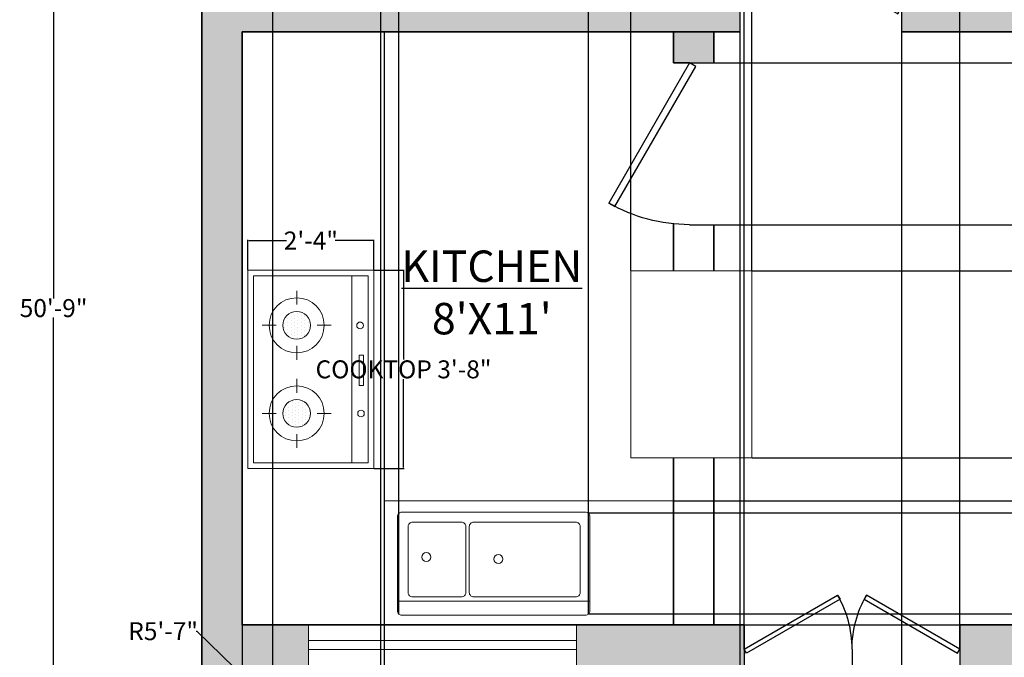
# Model space of a CAD drawing. Units: inches. Extents: x -37 to 408, y -619 to 75.
# Tile 2 of 4: x -37 to 182, y -354 to -212. Entities that reach past the tile are written whole.
import ezdxf

# ---------------------------------------------------------------- set-up
doc = ezdxf.new("R2010")
doc.units = ezdxf.units.IN
doc.header["$MEASUREMENT"] = 0
for name, color, linetype, lineweight in [('A-ANNO-DIMS', 2, 'Continuous', 18), ('A-AREA-IDEN', 7, 'Continuous', 25), ('A-DOOR', 4, 'Continuous', 25), ('A-EQPM', 9, 'Continuous', 18), ('A-FLOR-CASE', 8, 'Continuous', 18), ('A-FLOR-FIXT', 9, 'Continuous', 18), ('A-GLAZ', 4, 'Continuous', 18), ('A-WALL', 7, 'Continuous', 35), ('A-WALL-PATT', 16, 'Continuous', 13)]:
    doc.layers.add(name, color=color, linetype=linetype, lineweight=lineweight)
doc.styles.get("Standard").update_dxf_attribs({"font": 'arial.ttf'})
doc.dimstyles.get("Standard").update_dxf_attribs({"dimtxt": 4, "dimasz": 0.18, "dimexe": 0.18, "dimexo": 0.0625, "dimgap": 0.09, "dimtad": 0, "dimtih": 1, "dimtoh": 1, "dimdec": 1, "dimzin": 0, "dimdsep": 46, "dimlunit": 4, "dimtxsty": 'Standard', "dimcen": 0.09, "dimadec": 0, "dimazin": 0, "dimtfac": 1, "dimtdec": 1, "dimtofl": 0, "dimtmove": 0, "dimatfit": 3, "dimfxl": 1, "dimtolj": 1, "dimtzin": 0, "dimarcsym": 0})

# ---------------------------------------------------------------- blocks, each defined once
blk = doc.blocks.new('*U2')
for p, q in [((0, 0), (0, -6)), ((40, 0), (40, -6))]:
    blk.add_line(p, q)
blk.add_lwpolyline([(0, 0), (34.64, 20), (35.52, 18.48), (0.87, -1.52)], close=True)
blk.add_arc((0, 0), 40, 0, 30)
blk = doc.blocks.new('A$C475E21CF')
for p, q in [((0, 444.5), (0, 0)), ((0, 444.5), (699.9, 444.5)), ((19.4, 425), (19.4, 19.4)), ((19.4, 425), (680.5, 425)), ((680.5, 425), (680.5, 19.4)), ((699.9, 444.5), (699.9, 0)), ((194.5, 393.9), (194.5, 345.2)), ((505.4, 393.9), (505.4, 345.2)), ((498.4, 316.6), (498.4, 316.6)), ((510.6, 316.6), (510.6, 316.6)), ((522.7, 316.6), (522.7, 316.6)), ((160.9, 288.4), (160.9, 288.4)), ((166.9, 300.5), (166.9, 300.5)), ((173, 288.4), (173, 288.4)), ((179.1, 300.5), (179.1, 300.5)), ((185.2, 312.7), (185.2, 312.7)), ((185.2, 288.4), (185.2, 288.4)), ((191.2, 300.5), (191.2, 300.5)), ((197.3, 312.7), (197.3, 312.7)), ((197.3, 288.4), (197.3, 288.4)), ((203.4, 300.5), (203.4, 300.5)), ((209.5, 312.7), (209.5, 312.7)), ((209.5, 288.4), (209.5, 288.4)), ((215.6, 300.5), (215.6, 300.5)), ((221.6, 288.4), (221.6, 288.4)), ((227.7, 300.5), (227.7, 300.5)), ((233.8, 288.4), (233.8, 288.4)), ((468, 280.2), (468, 280.2)), ((474.1, 292.3), (474.1, 292.3)), ((480.2, 304.5), (480.2, 304.5)), ((480.2, 280.2), (480.2, 280.2)), ((486.3, 292.3), (486.3, 292.3)), ((492.3, 304.5), (492.3, 304.5)), ((492.3, 280.2), (492.3, 280.2)), ((498.4, 292.3), (498.4, 292.3)), ((504.5, 304.5), (504.5, 304.5)), ((504.5, 280.2), (504.5, 280.2)), ((510.6, 292.3), (510.6, 292.3)), ((516.7, 304.5), (516.7, 304.5)), ((516.7, 280.2), (516.7, 280.2)), ((522.7, 292.3), (522.7, 292.3)), ((528.8, 304.5), (528.8, 304.5)), ((528.8, 280.2), (528.8, 280.2)), ((534.9, 292.3), (534.9, 292.3)), ((541, 304.5), (541, 304.5)), ((541, 280.2), (541, 280.2)), ((547, 292.3), (547, 292.3)), ((553.1, 280.2), (553.1, 280.2)), ((72.9, 272.3), (121.6, 272.3)), ((148.7, 264.1), (148.7, 264.1)), ((154.8, 276.2), (154.8, 276.2)), ((154.8, 251.9), (154.8, 251.9)), ((160.9, 264.1), (160.9, 264.1)), ((166.9, 276.2), (166.9, 276.2)), ((166.9, 251.9), (166.9, 251.9)), ((173, 264.1), (173, 264.1)), ((179.1, 276.2), (179.1, 276.2)), ((179.1, 251.9), (179.1, 251.9)), ((185.2, 264.1), (185.2, 264.1)), ((191.2, 276.2), (191.2, 276.2)), ((191.2, 251.9), (191.2, 251.9)), ((197.3, 264.1), (197.3, 264.1)), ((203.4, 276.2), (203.4, 276.2)), ((203.4, 251.9), (203.4, 251.9)), ((209.5, 264.1), (209.5, 264.1)), ((215.6, 276.2), (215.6, 276.2)), ((215.6, 251.9), (215.6, 251.9)), ((221.6, 264.1), (221.6, 264.1)), ((227.7, 276.2), (227.7, 276.2)), ((227.7, 251.9), (227.7, 251.9)), ((233.8, 264.1), (233.8, 264.1)), ((239.9, 276.2), (239.9, 276.2)), ((239.9, 251.9), (239.9, 251.9)), ((267.4, 272.3), (316, 272.3)), ((383.9, 272.3), (432.5, 272.3)), ((462, 268), (462, 268)), ((468, 255.9), (468, 255.9)), ((474.1, 268), (474.1, 268)), ((474.1, 243.7), (474.1, 243.7)), ((480.2, 255.9), (480.2, 255.9)), ((486.3, 268), (486.3, 268)), ((486.3, 243.7), (486.3, 243.7)), ((492.3, 255.9), (492.3, 255.9)), ((498.4, 268), (498.4, 268)), ((498.4, 243.7), (498.4, 243.7)), ((504.5, 255.9), (504.5, 255.9)), ((510.6, 268), (510.6, 268)), ((510.6, 243.7), (510.6, 243.7)), ((516.7, 255.9), (516.7, 255.9)), ((522.7, 268), (522.7, 268)), ((522.7, 243.7), (522.7, 243.7)), ((528.8, 255.9), (528.8, 255.9)), ((534.9, 268), (534.9, 268)), ((534.9, 243.7), (534.9, 243.7)), ((541, 255.9), (541, 255.9)), ((547, 268), (547, 268)), ((547, 243.7), (547, 243.7)), ((553.1, 255.9), (553.1, 255.9)), ((578.4, 272.3), (627, 272.3)), ((160.9, 239.8), (160.9, 239.8)), ((173, 239.8), (173, 239.8)), ((179.1, 227.6), (179.1, 227.6)), ((185.2, 239.8), (185.2, 239.8)), ((191.2, 227.6), (191.2, 227.6)), ((197.3, 239.8), (197.3, 239.8)), ((203.4, 227.6), (203.4, 227.6)), ((209.5, 239.8), (209.5, 239.8)), ((215.6, 227.6), (215.6, 227.6)), ((221.6, 239.8), (221.6, 239.8)), ((233.8, 239.8), (233.8, 239.8)), ((492.3, 231.5), (492.3, 231.5)), ((504.5, 231.5), (504.5, 231.5)), ((516.7, 231.5), (516.7, 231.5)), ((528.8, 231.5), (528.8, 231.5)), ((194.5, 199.4), (194.5, 150.8)), ((505.4, 199.4), (505.4, 150.8)), ((19.4, 77.8), (680.5, 77.8)), ((293.4, 51.9), (400.6, 51.9)), ((293.4, 36.5), (293.4, 51.9)), ((400.6, 36.5), (293.4, 36.5)), ((400.6, 51.9), (400.6, 36.5)), ((0, 0), (699.9, 0)), ((19.4, 19.4), (680.5, 19.4))]:
    blk.add_line(p, q)
for centre, radius in [((194.5, 272.3), 97.2), ((505.4, 272.3), 97.2), ((194.5, 272.3), 48.6), ((505.4, 272.3), 48.6), ((193.9, 45.1), 11.7), ((505.2, 48.5), 11.7)]:
    blk.add_circle(centre, radius)
blk = doc.blocks.new('*D22')
at = {"layer": 'A-ANNO-DIMS', "color": 0, "lineweight": -2, "transparency": 16777216}
for p, q in [((41.93, -267.46), (48.67, -267.46)), ((48.49, -267.64), (48.49, -287.36)), ((48.49, -311.4), (48.49, -291.68)), ((41.93, -311.58), (48.67, -311.58))]:
    blk.add_line(p, q, dxfattribs=at)
at = {"layer": 'A-ANNO-DIMS', "color": 0, "transparency": 16777216}
for points in [[(48.46, -267.64), (48.52, -267.64), (48.49, -267.46)], [(48.46, -311.4), (48.52, -311.4), (48.49, -311.58)]]:
    blk.add_solid(points, dxfattribs=at)
at = {"layer": 'Defpoints', "color": 0, "transparency": 16777216}
for p in [(41.87, -267.46), (48.49, -267.46), (41.87, -311.58)]:
    blk.add_point(p, dxfattribs=at)
at = {"layer": 'A-ANNO-DIMS', "color": 0, "transparency": 16777216, "insert": (48.49, -289.52), "char_height": 4, "attachment_point": 5}
blk.add_mtext('\\A1;COOKTOP 3\'-8"', dxfattribs=at)
blk = doc.blocks.new('*D23')
at = {"layer": 'A-ANNO-DIMS', "color": 0, "lineweight": -2, "transparency": 16777216}
for p, q in [((13.85, -267.39), (13.85, -260.66)), ((14.03, -260.84), (22.42, -260.84)), ((41.69, -260.84), (33.3, -260.84)), ((41.87, -267.39), (41.87, -260.66))]:
    blk.add_line(p, q, dxfattribs=at)
at = {"layer": 'A-ANNO-DIMS', "color": 0, "transparency": 16777216}
for points in [[(14.03, -260.81), (14.03, -260.87), (13.85, -260.84)], [(41.69, -260.81), (41.69, -260.87), (41.87, -260.84)]]:
    blk.add_solid(points, dxfattribs=at)
at = {"layer": 'Defpoints', "color": 0, "transparency": 16777216}
for p in [(13.85, -260.84), (13.85, -267.46), (41.87, -267.46)]:
    blk.add_point(p, dxfattribs=at)
at = {"layer": 'A-ANNO-DIMS', "color": 0, "transparency": 16777216, "insert": (27.86, -260.84), "char_height": 4, "attachment_point": 5}
blk.add_mtext('\\A1;2\'-4"', dxfattribs=at)
blk = doc.blocks.new('*D28')
at = {"layer": 'A-ANNO-DIMS', "color": 0, "lineweight": -2, "transparency": 16777216}
for p, q in [((3.52, 28.62), (-29.6, 28.62)), ((-29.42, 28.44), (-29.42, -273.74)), ((-29.42, -580.2), (-29.42, -278.01)), ((3.52, -580.38), (-29.6, -580.38))]:
    blk.add_line(p, q, dxfattribs=at)
at = {"layer": 'A-ANNO-DIMS', "color": 0, "transparency": 16777216}
for points in [[(-29.45, 28.44), (-29.39, 28.44), (-29.42, 28.62)], [(-29.45, -580.2), (-29.39, -580.2), (-29.42, -580.38)]]:
    blk.add_solid(points, dxfattribs=at)
at = {"layer": 'Defpoints', "color": 0, "transparency": 16777216}
for p in [(-29.42, 28.62), (3.58, 28.62), (3.58, -580.38)]:
    blk.add_point(p, dxfattribs=at)
at = {"layer": 'A-ANNO-DIMS', "color": 0, "transparency": 16777216, "insert": (-29.42, -275.88), "char_height": 4, "attachment_point": 5}
blk.add_mtext('\\A1;50\'-9"', dxfattribs=at)
blk = doc.blocks.new('*D34')
at = {"layer": 'A-ANNO-DIMS', "color": 0, "lineweight": -2, "transparency": 16777216}
for p, q in [((124.36, -346.31), (124.36, 69.37)), ((124.54, 69.19), (142.88, 69.19)), ((172.18, 69.19), (153.85, 69.19)), ((172.36, -346.31), (172.36, 69.37))]:
    blk.add_line(p, q, dxfattribs=at)
at = {"layer": 'A-ANNO-DIMS', "color": 0, "transparency": 16777216}
for points in [[(124.54, 69.22), (124.54, 69.16), (124.36, 69.19)], [(172.18, 69.22), (172.18, 69.16), (172.36, 69.19)]]:
    blk.add_solid(points, dxfattribs=at)
at = {"layer": 'Defpoints', "color": 0, "transparency": 16777216}
for p in [(172.36, 69.19), (124.36, -346.38), (172.36, -346.38)]:
    blk.add_point(p, dxfattribs=at)
at = {"layer": 'A-ANNO-DIMS', "color": 0, "transparency": 16777216, "insert": (148.36, 69.19), "char_height": 4, "attachment_point": 5}
blk.add_mtext('\\A1;4\'-0"', dxfattribs=at)
blk = doc.blocks.new('*D37')
at = {"layer": 'A-ANNO-DIMS', "color": 0, "lineweight": -2, "transparency": 16777216}
for p, q in [((12.58, -214.44), (12.58, -613.56)), ((44.21, -214.44), (44.21, -613.56)), ((12.76, -613.38), (18.3, -613.38)), ((44.03, -613.38), (38.5, -613.38))]:
    blk.add_line(p, q, dxfattribs=at)
at = {"layer": 'A-ANNO-DIMS', "color": 0, "transparency": 16777216}
for points in [[(12.76, -613.35), (12.76, -613.41), (12.58, -613.38)], [(44.03, -613.35), (44.03, -613.41), (44.21, -613.38)]]:
    blk.add_solid(points, dxfattribs=at)
at = {"layer": 'Defpoints', "color": 0, "transparency": 16777216}
for p in [(12.58, -214.38), (44.21, -214.38), (44.21, -613.38)]:
    blk.add_point(p, dxfattribs=at)
at = {"layer": 'A-ANNO-DIMS', "color": 0, "transparency": 16777216, "insert": (28.4, -613.38), "char_height": 4, "attachment_point": 5}
blk.add_mtext('\\A1;2\'-7 1/2"', dxfattribs=at)
blk = doc.blocks.new('*D38')
at = {"layer": 'A-ANNO-DIMS', "color": 0, "lineweight": -2, "transparency": 16777216}
for p, q in [((123.34, -214.44), (123.34, -613.56)), ((159.34, -214.44), (159.34, -613.56)), ((123.52, -613.38), (135.93, -613.38)), ((159.16, -613.38), (146.74, -613.38))]:
    blk.add_line(p, q, dxfattribs=at)
at = {"layer": 'A-ANNO-DIMS', "color": 0, "transparency": 16777216}
for points in [[(123.52, -613.35), (123.52, -613.41), (123.34, -613.38)], [(159.16, -613.35), (159.16, -613.41), (159.34, -613.38)]]:
    blk.add_solid(points, dxfattribs=at)
at = {"layer": 'Defpoints', "color": 0, "transparency": 16777216}
for p in [(123.34, -214.38), (159.34, -214.38), (159.34, -613.38)]:
    blk.add_point(p, dxfattribs=at)
at = {"layer": 'A-ANNO-DIMS', "color": 0, "transparency": 16777216, "insert": (141.34, -613.38), "char_height": 4, "attachment_point": 5}
blk.add_mtext('\\A1;3\'-0"', dxfattribs=at)
blk = doc.blocks.new('*D39')
at = {"layer": 'A-ANNO-DIMS', "color": 0, "lineweight": -2, "transparency": 16777216}
for p, q in [((19.34, -49.44), (19.34, -613.56)), ((43.34, -49.44), (43.34, -613.56)), ((19.52, -613.38), (25.9, -613.38)), ((43.16, -613.38), (36.78, -613.38))]:
    blk.add_line(p, q, dxfattribs=at)
at = {"layer": 'A-ANNO-DIMS', "color": 0, "transparency": 16777216}
for points in [[(19.52, -613.35), (19.52, -613.41), (19.34, -613.38)], [(43.16, -613.35), (43.16, -613.41), (43.34, -613.38)]]:
    blk.add_solid(points, dxfattribs=at)
at = {"layer": 'Defpoints', "color": 0, "transparency": 16777216}
for p in [(19.34, -49.38), (43.34, -49.38), (43.34, -613.38)]:
    blk.add_point(p, dxfattribs=at)
at = {"layer": 'A-ANNO-DIMS', "color": 0, "transparency": 16777216, "insert": (31.34, -613.38), "char_height": 4, "attachment_point": 5}
blk.add_mtext('\\A1;2\'-0"', dxfattribs=at)
blk = doc.blocks.new('*D43')
at = {"layer": 'A-ANNO-DIMS', "color": 0, "lineweight": -2, "transparency": 16777216}
for p, q in [((47.42, -343.92), (47.42, 69.37)), ((47.6, 69.19), (58.49, 69.19)), ((89.51, 69.19), (78.62, 69.19)), ((89.69, -343.92), (89.69, 69.37))]:
    blk.add_line(p, q, dxfattribs=at)
at = {"layer": 'A-ANNO-DIMS', "color": 0, "transparency": 16777216}
for points in [[(47.6, 69.22), (47.6, 69.16), (47.42, 69.19)], [(89.51, 69.22), (89.51, 69.16), (89.69, 69.19)]]:
    blk.add_solid(points, dxfattribs=at)
at = {"layer": 'Defpoints', "color": 0, "transparency": 16777216}
for p in [(89.69, 69.19), (47.42, -343.98), (89.69, -343.98)]:
    blk.add_point(p, dxfattribs=at)
at = {"layer": 'A-ANNO-DIMS', "color": 0, "transparency": 16777216, "insert": (68.55, 69.19), "char_height": 4, "attachment_point": 5}
blk.add_mtext('\\A1;3\'-6 1/2"', dxfattribs=at)
blk = doc.blocks.new('*D44')
at = {"layer": 'A-ANNO-DIMS', "color": 0, "lineweight": -2, "transparency": 16777216}
for p, q in [((89.6, -321.48), (396.76, -321.48)), ((396.58, -321.66), (396.58, -330.57)), ((396.58, -343.8), (396.58, -334.89)), ((89.76, -343.98), (396.76, -343.98))]:
    blk.add_line(p, q, dxfattribs=at)
at = {"layer": 'A-ANNO-DIMS', "color": 0, "transparency": 16777216}
for points in [[(396.55, -321.66), (396.61, -321.66), (396.58, -321.48)], [(396.55, -343.8), (396.61, -343.8), (396.58, -343.98)]]:
    blk.add_solid(points, dxfattribs=at)
at = {"layer": 'Defpoints', "color": 0, "transparency": 16777216}
for p in [(89.54, -321.48), (396.58, -321.48), (89.69, -343.98)]:
    blk.add_point(p, dxfattribs=at)
at = {"layer": 'A-ANNO-DIMS', "color": 0, "transparency": 16777216, "insert": (396.58, -332.73), "char_height": 4, "attachment_point": 5}
blk.add_mtext('\\A1;1\'-10 1/2"', dxfattribs=at)
blk = doc.blocks.new('*D45')
at = {"layer": 'A-ANNO-DIMS', "color": 0, "lineweight": -2, "transparency": 16777216}
for p, q in [((117.64, -221.31), (396.76, -221.31)), ((396.58, -221.49), (396.58, -237.17)), ((396.58, -257.13), (396.58, -241.44)), ((117.64, -257.31), (396.76, -257.31))]:
    blk.add_line(p, q, dxfattribs=at)
at = {"layer": 'A-ANNO-DIMS', "color": 0, "transparency": 16777216}
for points in [[(396.55, -221.49), (396.61, -221.49), (396.58, -221.31)], [(396.55, -257.13), (396.61, -257.13), (396.58, -257.31)]]:
    blk.add_solid(points, dxfattribs=at)
at = {"layer": 'Defpoints', "color": 0, "transparency": 16777216}
for p in [(117.58, -221.31), (396.58, -221.31), (117.58, -257.31)]:
    blk.add_point(p, dxfattribs=at)
at = {"layer": 'A-ANNO-DIMS', "color": 0, "transparency": 16777216, "insert": (396.58, -239.31), "char_height": 4, "attachment_point": 5}
blk.add_mtext('\\A1;3\'-0"', dxfattribs=at)
blk = doc.blocks.new('*D46')
at = {"layer": 'A-ANNO-DIMS', "color": 0, "lineweight": -2, "transparency": 16777216}
for p, q in [((108.64, -318.81), (396.76, -318.81)), ((396.58, -318.99), (396.58, -330.43)), ((396.58, -346.2), (396.58, -334.75)), ((108.64, -346.38), (396.76, -346.38))]:
    blk.add_line(p, q, dxfattribs=at)
at = {"layer": 'A-ANNO-DIMS', "color": 0, "transparency": 16777216}
for points in [[(396.55, -318.99), (396.61, -318.99), (396.58, -318.81)], [(396.55, -346.2), (396.61, -346.2), (396.58, -346.38)]]:
    blk.add_solid(points, dxfattribs=at)
at = {"layer": 'Defpoints', "color": 0, "transparency": 16777216}
for p in [(108.58, -318.81), (108.58, -346.38), (396.58, -346.38)]:
    blk.add_point(p, dxfattribs=at)
at = {"layer": 'A-ANNO-DIMS', "color": 0, "transparency": 16777216, "insert": (396.58, -332.59), "char_height": 4, "attachment_point": 5}
blk.add_mtext('\\A1;2\'-3 1/2"', dxfattribs=at)
blk = doc.blocks.new('*D52')
at = {"layer": 'A-ANNO-DIMS', "color": 0, "lineweight": -2, "transparency": 16777216}
for p, q in [((126.12, -267.56), (396.76, -267.56)), ((396.58, -267.74), (396.58, -286.24)), ((396.58, -309.05), (396.58, -290.56)), ((126.12, -309.23), (396.76, -309.23))]:
    blk.add_line(p, q, dxfattribs=at)
at = {"layer": 'A-ANNO-DIMS', "color": 0, "transparency": 16777216}
for points in [[(396.55, -267.74), (396.61, -267.74), (396.58, -267.56)], [(396.55, -309.05), (396.61, -309.05), (396.58, -309.23)]]:
    blk.add_solid(points, dxfattribs=at)
at = {"layer": 'Defpoints', "color": 0, "transparency": 16777216}
for p in [(126.06, -267.56), (126.06, -309.23), (396.58, -309.23)]:
    blk.add_point(p, dxfattribs=at)
at = {"layer": 'A-ANNO-DIMS', "color": 0, "transparency": 16777216, "insert": (396.58, -288.4), "char_height": 4, "attachment_point": 5}
blk.add_mtext('\\A1;3\'-5 1/2"', dxfattribs=at)
blk = doc.blocks.new('*D53')
at = {"layer": 'A-ANNO-DIMS', "color": 0, "lineweight": -2, "transparency": 16777216}
for p, q in [((99.07, -267.5), (99.07, 69.37)), ((99.25, 69.19), (107.12, 69.19)), ((125.88, 69.19), (118, 69.19)), ((126.06, -267.5), (126.06, 69.37))]:
    blk.add_line(p, q, dxfattribs=at)
at = {"layer": 'A-ANNO-DIMS', "color": 0, "transparency": 16777216}
for points in [[(99.25, 69.22), (99.25, 69.16), (99.07, 69.19)], [(125.88, 69.22), (125.88, 69.16), (126.06, 69.19)]]:
    blk.add_solid(points, dxfattribs=at)
at = {"layer": 'Defpoints', "color": 0, "transparency": 16777216}
for p in [(126.06, 69.19), (99.07, -267.56), (126.06, -267.56)]:
    blk.add_point(p, dxfattribs=at)
at = {"layer": 'A-ANNO-DIMS', "color": 0, "transparency": 16777216, "insert": (112.56, 69.19), "char_height": 4, "attachment_point": 5}
blk.add_mtext('\\A1;2\'-3"', dxfattribs=at)
blk = doc.blocks.new('*D54')
at = {"layer": 'A-ANNO-DIMS', "color": 0, "lineweight": -2, "transparency": 16777216}
for p, q in [((2.29, -347.81), (2.47, -347.81)), ((2.47, -347.81), (31.34, -375.72)), ((79.72, -422.57), (79.9, -422.57)), ((79.81, -422.66), (79.81, -422.48))]:
    blk.add_line(p, q, dxfattribs=at)
at = {"layer": 'A-ANNO-DIMS', "color": 0, "transparency": 16777216}
blk.add_solid([(31.36, -375.7), (31.32, -375.74), (31.47, -375.84)], dxfattribs=at)
at = {"layer": 'Defpoints', "color": 0, "transparency": 16777216}
for p in [(31.47, -375.84), (79.81, -422.57)]:
    blk.add_point(p, dxfattribs=at)
at = {"layer": 'A-ANNO-DIMS', "color": 0, "transparency": 16777216, "insert": (-5.03, -347.81), "char_height": 4, "attachment_point": 5}
blk.add_mtext('\\A1;R5\'-7"', dxfattribs=at)

msp = doc.modelspace()

# ---------------------------------------------------------------- hatches: boundary and pattern name
at = {"layer": 'A-WALL-PATT'}
h = msp.add_hatch(color=256, dxfattribs=at)
h.dxf.hatch_style = 1
h.paths.add_polyline_path([(117.58, 28.62), (3.58, 28.62), (3.58, -49.38), (19.34, -49.38), (19.34, -45.78), (19.34, -44.88), (12.58, -44.88), (12.58, 19.62), (108.58, 19.62), (108.58, 5.94), (117.58, 5.94), (117.58, 19.62)])
h.paths.add_polyline_path([(363.58, 28.62), (261.58, 28.62), (261.58, 19.62), (261.58, 6.04), (265.18, 6.04, -0.056797), (270.58, 5.42), (270.58, 19.62), (354.58, 19.62), (354.58, -44.88), (363.58, -44.88)])
h.paths.add_polyline_path([(124.92, -40.38), (117.58, -40.38), (117.58, -20.71), (108.58, -20.71), (108.58, -44.88), (43.33, -44.88, -0.009377), (43.34, -45.78), (43.34, -49.38), (124.92, -49.38)])
h.paths.add_polyline_path([(209.99, -40.38), (164.76, -40.38), (164.76, -49.38), (209.99, -49.38)])
h.paths.add_polyline_path([(270.58, -17.96), (265.18, -17.96), (261.58, -17.96), (261.58, -40.38), (252.1, -40.38, -0.056797), (252.72, -45.78), (252.72, -49.38), (354.58, -49.38), (354.58, -205.38), (363.58, -205.38), (363.58, -44.88), (354.58, -44.88), (270.58, -44.88)])
h.paths.add_polyline_path([(12.58, -49.38), (3.58, -49.38), (3.58, -205.38), (12.58, -205.38)])
h.paths.add_polyline_path([(205.47, -208.98), (205.47, -205.38), (159.34, -205.38), (159.34, -208.98), (159.34, -214.38), (205.47, -214.38)])
h = msp.add_hatch(color=256, dxfattribs=at)
h.dxf.hatch_style = 1
h.paths.add_polyline_path([(123.52, -205.38), (3.58, -205.38), (3.58, -355.38), (27.35, -355.38), (27.35, -346.38), (12.58, -346.38), (12.58, -214.38), (123.34, -214.38), (123.34, -208.98, -0.025047)])
h.paths.add_polyline_path([(117.58, -214.38), (108.58, -214.38), (108.58, -221.31), (112.18, -221.31), (117.58, -221.31)], flags=17)
h.paths.add_polyline_path([(124.36, -346.38), (86.98, -346.38), (86.98, -355.38), (124.36, -355.38), (124.36, -351.78)])
h.paths.add_polyline_path([(222.97, -346.38), (172.36, -346.38), (172.36, -351.78), (172.36, -355.38), (180.58, -355.38), (180.58, -364.83), (185.98, -364.83), (189.58, -364.83), (189.58, -355.38), (222.97, -355.38)])
h.paths.add_polyline_path([(363.58, -205.38), (241.29, -205.38, -0.025047), (241.47, -208.98), (241.47, -214.38), (354.58, -214.38), (354.58, -346.38), (317.68, -346.38), (317.68, -355.38), (363.58, -355.38)])

# ---------------------------------------------------------------- linework, layer by layer
at = {"layer": 'A-FLOR-CASE'}
for p, q in [((44.21, -214.38), (44.21, -318.81)), ((126.06, -267.56), (99.07, -267.56)), ((99.07, -267.56), (99.07, -309.23)), ((126.06, -309.23), (126.06, -267.56)), ((99.07, -309.23), (126.06, -309.23)), ((44.21, -318.81), (108.58, -318.81))]:
    msp.add_line(p, q, dxfattribs=at)
at = {"layer": 'A-FLOR-FIXT'}
msp.add_line((47.12, -341.13), (89.99, -341.13), dxfattribs=at)
for points in [[(48.12, -321.31), (88.99, -321.31, -0.414214), (89.99, -322.31), (89.99, -343.28, -0.414214), (88.99, -344.28), (48.12, -344.28, -0.414214), (47.12, -343.28), (47.12, -322.31, -0.414214)], [(50.51, -323.51), (61.36, -323.51, -0.414214), (62.36, -324.51), (62.36, -339.2, -0.414214), (61.36, -340.2), (50.51, -340.2, -0.414214), (49.51, -339.2), (49.51, -324.51, -0.414214)], [(64.13, -323.51), (86.81, -323.51, -0.414214), (87.81, -324.51), (87.81, -339.2, -0.414214), (86.81, -340.2), (64.13, -340.2, -0.414214), (63.13, -339.2), (63.13, -324.51, -0.414214)]]:
    msp.add_lwpolyline(points, format="xyb", close=True, dxfattribs=at)
for centre in [(53.57, -331.31), (69.62, -331.76)]:
    msp.add_circle(centre, 0.989, dxfattribs=at)
at = {"layer": 'A-GLAZ'}
for p, q in [((27.35, -346.38), (27.35, -355.38)), ((86.98, -346.38), (86.98, -355.38)), ((27.35, -349.88), (86.98, -349.88)), ((27.35, -351.88), (86.98, -351.88))]:
    msp.add_line(p, q, dxfattribs=at)
at = {"layer": 'A-WALL'}
for p, q in [((3.58, 28.62), (3.58, -580.38)), ((12.58, -214.38), (123.34, -214.38)), ((12.58, -214.38), (12.58, -346.38)), ((108.58, -214.38), (108.58, -221.31)), ((117.58, -214.38), (117.58, -221.31)), ((159.34, -214.38), (205.47, -214.38)), ((112.18, -221.31), (108.58, -221.31)), ((108.58, -257.13), (108.58, -267.56)), ((117.58, -257.31), (117.58, -267.56)), ((108.58, -309.23), (108.58, -346.38)), ((117.58, -309.23), (117.58, -346.38)), ((12.58, -346.38), (124.36, -346.38)), ((124.36, -351.78), (124.36, -346.38)), ((172.36, -351.78), (172.36, -346.38)), ((172.36, -346.38), (222.97, -346.38))]:
    msp.add_line(p, q, dxfattribs=at)

# ---------------------------------------------------------------- block references
at = {"layer": 'A-DOOR'}
for p, xscale, yscale, zscale in [((159.34, -208.98), -0.9, 0.9, 0.9), ((124.36, -351.78), 0.6, 0.6, 0.6), ((172.36, -351.78), -0.6, 0.6, 0.6)]:
    msp.add_blockref('*U2', p, dxfattribs=dict(at, xscale=xscale, yscale=yscale, zscale=zscale))
at = {"layer": 'A-DOOR', "xscale": -0.9, "yscale": 0.9, "zscale": 0.9, "rotation": 90}
msp.add_blockref('*U2', (112.18, -221.31), dxfattribs=at)
at = {"layer": 'A-EQPM', "xscale": 0.0630415206883198, "yscale": 0.0630415206883198, "zscale": 0.0630415206883198, "rotation": 89.99999999999999}
msp.add_blockref('A$C475E21CF', (41.87, -311.58), dxfattribs=at)

# ---------------------------------------------------------------- texts
at = {"layer": 'A-AREA-IDEN', "insert": (39.57, -263.06), "char_height": 7, "attachment_point": 1}
msp.add_mtext_dynamic_manual_height_columns("\\A1;\\pxqc;{\\fArial|b1|i0|c0|p34;\\LKITCHEN\\P\\l8'X11'}", width=57.1656, gutter_width=1, heights=[0], dxfattribs=at)

# ---------------------------------------------------------------- dimensions: what is measured, and where the dimension line sits
at = {"layer": 'A-ANNO-DIMS'}
for base, p1, p2, picture, middle in [((89.69, 69.19), (47.42, -343.98), (89.69, -343.98), '*D43', (68.55, 69.19)), ((126.06, 69.19), (99.07, -267.56), (126.06, -267.56), '*D53', (112.56, 69.19)), ((172.36, 69.19), (124.36, -346.38), (172.36, -346.38), '*D34', (148.36, 69.19)), ((43.34, -613.38), (19.34, -49.38), (43.34, -49.38), '*D39', (31.34, -613.38)), ((44.21, -613.38), (12.58, -214.38), (44.21, -214.38), '*D37', (28.4, -613.38)), ((159.34, -613.38), (123.34, -214.38), (159.34, -214.38), '*D38', (141.34, -613.38))]:
    dim = msp.add_linear_dim(base=base, p1=p1, p2=p2, dimstyle='Standard', override={"dimdec": 1, "dimlfac": 1, "dimrnd": 0, "dimzin": 1, "dimdsep": 46, "dimlunit": 4, "dimfrac": 2}, dxfattribs=at)
    dim.commit()
    dim.dimension.update_dxf_attribs({"geometry": picture, "text_midpoint": middle})
for base, p1, p2, angle, picture, middle in [((-29.42, 28.62), (3.58, -580.38), (3.58, 28.62), 90, '*D28', (-29.42, -275.88)), ((396.58, -221.31), (117.58, -257.31), (117.58, -221.31), 90, '*D45', (396.58, -239.31)), ((13.85, -260.84), (41.87, -267.46), (13.85, -267.46), 180, '*D23', (27.86, -260.84)), ((396.58, -309.23), (126.06, -267.56), (126.06, -309.23), 90, '*D52', (396.58, -288.4)), ((396.58, -346.38), (108.58, -318.81), (108.58, -346.38), 90, '*D46', (396.58, -332.59)), ((396.58, -321.48), (89.69, -343.98), (89.54, -321.48), 90, '*D44', (396.58, -332.73))]:
    dim = msp.add_linear_dim(base=base, p1=p1, p2=p2, angle=angle, dimstyle='Standard', override={"dimdec": 1, "dimlfac": 1, "dimrnd": 0, "dimzin": 1, "dimdsep": 46, "dimlunit": 4, "dimfrac": 2}, dxfattribs=at)
    dim.commit()
    dim.dimension.update_dxf_attribs({"geometry": picture, "text_midpoint": middle})
dim = msp.add_linear_dim(base=(48.49, -267.46), p1=(41.87, -311.58), p2=(41.87, -267.46), angle=90, text='COOKTOP <>', dimstyle='Standard', override={"dimdec": 1, "dimlfac": 1, "dimrnd": 0, "dimzin": 1, "dimdsep": 46, "dimlunit": 4, "dimfrac": 2}, dxfattribs=at)
dim.commit()
dim.dimension.update_dxf_attribs({"geometry": '*D22', "text_midpoint": (48.49, -289.52)})
dim = msp.add_radius_dim(center=(79.81, -422.57), mpoint=(31.47, -375.84), dimstyle='Standard', override={"dimdec": 1, "dimlfac": 1, "dimrnd": 0, "dimzin": 1, "dimdsep": 46, "dimlunit": 4, "dimfrac": 2}, dxfattribs=at)
dim.commit()
dim.dimension.update_dxf_attribs({"geometry": '*D54', "text_midpoint": (-5.03, -347.81), "dimtype": 164})

doc.saveas('drawing.dxf')
